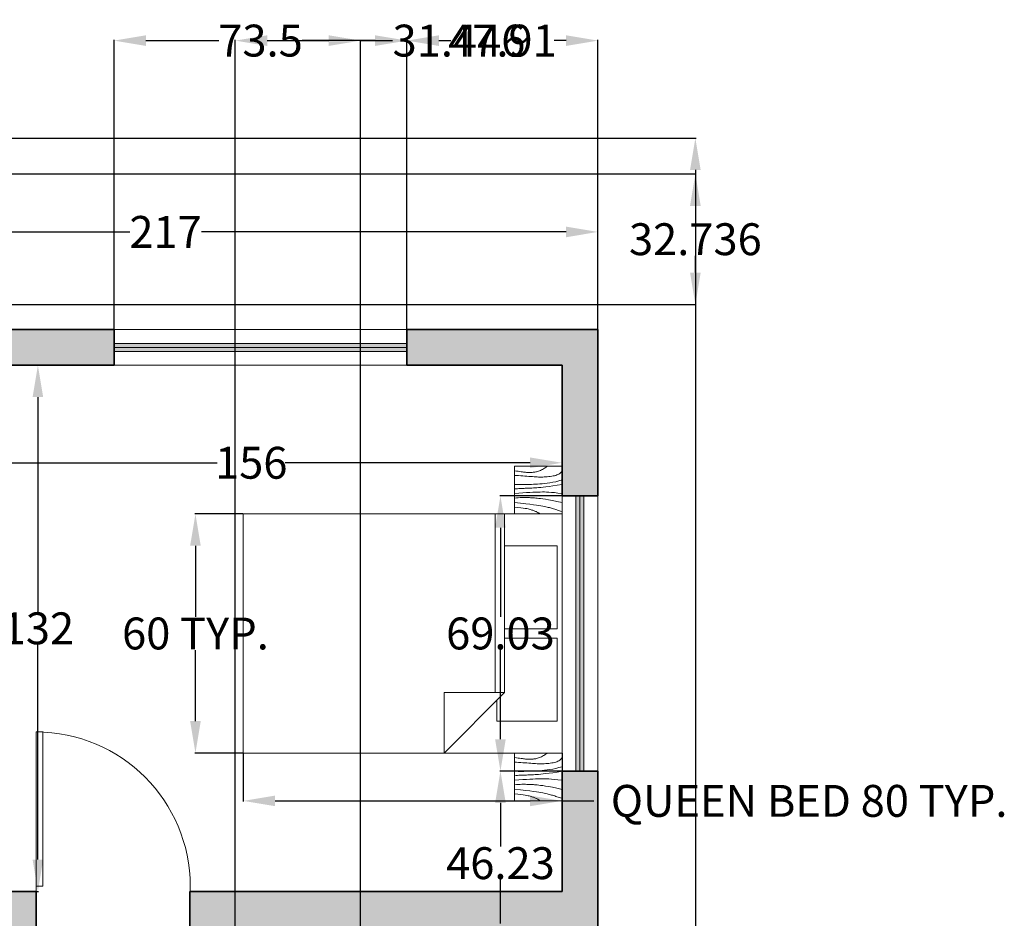
# Model space of a CAD drawing. Units: inches. Extents: x -52 to 678, y 23 to 685.
# Tile 11 of 11: x 431 to 678, y 329 to 555. Entities that reach past the tile are written whole.
import ezdxf

# ---------------------------------------------------------------- set-up
doc = ezdxf.new("R2010")
doc.units = ezdxf.units.IN
doc.header["$MEASUREMENT"] = 0
for name, color, linetype, lineweight in [('A-ANNO-DIMS', 2, 'Continuous', 18), ('A-DOOR', 3, 'Continuous', 18), ('A-FURN', 8, 'Continuous', 18), ('A-GLAZ', 4, 'Continuous', 18), ('A-WALL', 7, 'Continuous', 35)]:
    doc.layers.add(name, color=color, linetype=linetype, lineweight=lineweight)
doc.layers.add('A-GLAZ-PATT', color=18, linetype='Continuous', lineweight=13, true_color=0x000000)
doc.layers.add('A-WALL-PATT', color=18, linetype='Continuous', lineweight=13, true_color=0x000000)
doc.styles.get("Standard").update_dxf_attribs({"font": 'arial.ttf'})
doc.dimstyles.get("Standard").update_dxf_attribs({"dimtxt": 8, "dimasz": 8, "dimexe": 0.18, "dimexo": 0.0625, "dimgap": 0.09, "dimtad": 0, "dimtih": 1, "dimtoh": 1, "dimdec": 0, "dimzin": 0, "dimdsep": 46, "dimlunit": 3, "dimtxsty": 'Standard', "dimcen": 0.09, "dimadec": 0, "dimazin": 0, "dimtfac": 1, "dimtdec": 0, "dimtofl": 0, "dimtmove": 0, "dimatfit": 3, "dimfxl": 1, "dimtolj": 1, "dimtzin": 0, "dimarcsym": 0})

# ---------------------------------------------------------------- blocks, each defined once
blk = doc.blocks.new('Table - Square Woodgrain 42 x 42 in.')
blk.add_line((0, -42), (42, -42))
for points in [[(0, -4), (1.704, -4.2172), (3.2358, -4.4188), (4.615, -4.604), (5.8615, -4.7721), (6.9951, -4.9224), (8.0357, -5.0541), (9.0031, -5.1667), (9.9171, -5.2594), (10.7951, -5.3316), (11.6445, -5.3836), (12.4702, -5.4157), (13.277, -5.4283), (14.0698, -5.4217), (14.8535, -5.3964), (15.6331, -5.3526), (16.4133, -5.2908), (17.1986, -5.2103), (17.9913, -5.1062), (18.793, -4.9727), (19.6056, -4.8038), (20.4307, -4.5937), (21.2701, -4.3365), (22.1256, -4.0262), (22.9989, -3.6571), (23.888, -3.2272), (24.7756, -2.7516), (25.6408, -2.2491), (26.4624, -1.7387), (27.2195, -1.2395), (27.891, -0.7703), (28.456, -0.3501), (28.8934, 0.002)], [(0, -42), (0, 0), (42, 0), (42, -42)], [(0, -8), (1.8203, -8.1001), (3.6741, -8.2149), (5.5411, -8.3408), (7.4011, -8.4741), (9.2339, -8.6112), (11.0193, -8.7484), (12.7371, -8.8821), (14.3671, -9.0086), (15.8954, -9.1246), (17.3337, -9.2278), (18.6997, -9.3159), (20.0116, -9.387), (21.2871, -9.4389), (22.5442, -9.4696), (23.8008, -9.477), (25.0749, -9.459), (26.3791, -9.4137), (27.7049, -9.3403), (29.0383, -9.2382), (30.3655, -9.1068), (31.6728, -8.9455), (32.9461, -8.7535), (34.1717, -8.5304), (35.3358, -8.2756), (36.4268, -7.9863), (37.443, -7.6521), (38.3849, -7.2603), (39.253, -6.7986), (40.048, -6.2542), (40.7705, -5.6147), (41.421, -4.8674), (42, -4)], [(42, -12), (39.1784, -12.8621), (36.4519, -13.5654), (33.8246, -14.1294), (31.3004, -14.5731), (28.8832, -14.9161), (26.577, -15.1775), (24.3858, -15.3768), (22.3136, -15.5332), (20.3622, -15.6632), (18.5254, -15.7718), (16.7947, -15.8612), (15.1618, -15.9338), (13.6183, -15.9916), (12.1558, -16.0369), (10.7659, -16.0718), (9.4403, -16.0987), (8.1703, -16.1191), (6.9461, -16.1325), (5.7577, -16.1377), (4.595, -16.1335), (3.4479, -16.1188), (2.3064, -16.0924), (1.1604, -16.0532), (0, -16)], [(42, -16), (37.6529, -16.7365), (33.8802, -17.329), (30.6179, -17.7961), (27.8015, -18.1561), (25.3668, -18.4275), (23.2497, -18.6288), (21.3859, -18.7785), (19.7111, -18.8949), (18.1693, -18.9939), (16.7375, -19.0795), (15.401, -19.1534), (14.1449, -19.217), (12.9544, -19.2717), (11.8148, -19.3191), (10.7113, -19.3606), (9.6291, -19.3976), (8.5534, -19.4323), (7.47, -19.4689), (6.3643, -19.5122), (5.222, -19.5672), (4.0288, -19.6386), (2.7703, -19.7313), (1.4321, -19.8501), (0, -20)], [(0, -24), (3.9243, -23.6805), (7.4766, -23.4138), (10.6891, -23.1954), (13.5943, -23.0205), (16.2247, -22.8847), (18.6125, -22.7832), (20.7903, -22.7116), (22.7903, -22.6651), (24.6563, -22.642), (26.4764, -22.6507), (28.35, -22.7024), (30.3766, -22.8084), (32.6555, -22.98), (35.2861, -23.2283), (38.3678, -23.5645), (42, -24)], [(42, -32), (37.392, -31.017), (33.4585, -30.2231), (30.1291, -29.5949), (27.3334, -29.109), (25.0009, -28.742), (23.0612, -28.4707), (21.4439, -28.2716), (20.0786, -28.1215), (18.8998, -28.0002), (17.8609, -27.9014), (16.9206, -27.8219), (16.0371, -27.7588), (15.1691, -27.709), (14.2748, -27.6693), (13.3128, -27.6368), (12.2415, -27.6083), (11.0295, -27.5824), (9.6867, -27.5643), (8.233, -27.5608), (6.6884, -27.5787), (5.0728, -27.6248), (3.4062, -27.7058), (1.7086, -27.8286), (0, -28)], [(0, -32), (5.4026, -32.5358), (9.9494, -33.019), (13.7424, -33.4553), (16.8834, -33.8505), (19.4743, -34.2106), (21.6171, -34.5413), (23.4136, -34.8486), (24.9657, -35.1382), (26.3614, -35.4156), (27.6332, -35.6841), (28.7995, -35.9467), (29.8788, -36.2064), (30.8897, -36.4661), (31.8507, -36.7288), (32.7802, -36.9973), (33.6968, -37.2747), (34.6175, -37.5635), (35.5531, -37.8651), (36.5128, -38.1805), (37.506, -38.5108), (38.5421, -38.8568), (39.6302, -39.2197), (40.7797, -39.6004), (42, -40)], [(0, -36), (3.0098, -36.2857), (5.5354, -36.5643), (7.6368, -36.8359), (9.374, -37.1009), (10.807, -37.3597), (11.9957, -37.6126), (13.0002, -37.8599), (13.8804, -38.102), (14.6874, -38.3393), (15.4365, -38.5729), (16.1338, -38.8041), (16.7858, -39.0341), (17.3987, -39.264), (17.9787, -39.4952), (18.5322, -39.7288), (19.0655, -39.9662), (19.5832, -40.2081), (20.0842, -40.4544), (20.5657, -40.7046), (21.0249, -40.9581), (21.459, -41.2144), (21.8653, -41.4731), (22.2409, -41.7335), (22.5831, -41.9951)]]:
    blk.add_lwpolyline(points)
blk = doc.blocks.new('*U14')
for p, q in [((0, 0), (0, -6)), ((40, 0), (40, -6))]:
    blk.add_line(p, q)
blk.add_lwpolyline([(0, 0), (0, 40), (1.75, 40), (1.75, 0)], close=True)
blk.add_arc((0, 0), 40, 0, 90)
blk = doc.blocks.new('Bed - Queen')
for p, q in [((0, -80.00003), (0, 0)), ((0, 0), (59.99999, 0)), ((59.99999, 0), (59.99999, -80.00003)), ((7.99999, -1.2), (28.79998, -1.2)), ((7.99999, -14.4), (7.99999, -1.2)), ((28.79998, -1.2), (28.79998, -14.4)), ((31.19999, -1.2), (51.99999, -1.2)), ((31.19999, -14.4), (31.19999, -1.2)), ((51.99999, -1.2), (51.99999, -16.4)), ((0, -14.4), (44.8, -14.4)), ((59.99999, -29.6), (44.8, -14.4)), ((44.8, -14.4), (44.8, -29.6)), ((44.8, -16.8), (0, -16.8)), ((51.99999, -16.4), (46.79936, -16.4)), ((44.8, -29.6), (59.99999, -29.6)), ((59.99999, -80.00003), (0, -80.00003))]:
    blk.add_line(p, q)
blk = doc.blocks.new('*D19')
at = {"layer": 'A-ANNO-DIMS', "color": 0, "lineweight": -2, "transparency": 16777216}
for p, q in [((486.61, 370.77), (486.61, 358.66)), ((566.61, 370.77), (566.61, 358.66)), ((494.61, 358.84), (558.61, 358.84)), ((566.61, 358.84), (574.61, 358.84))]:
    blk.add_line(p, q, dxfattribs=at)
at = {"layer": 'A-ANNO-DIMS', "color": 0, "transparency": 16777216}
for points in [[(494.61, 360.17), (494.61, 357.5), (486.61, 358.84)], [(558.61, 360.17), (558.61, 357.5), (566.61, 358.84)]]:
    blk.add_solid(points, dxfattribs=at)
at = {"layer": 'Defpoints', "color": 0, "transparency": 16777216}
for p in [(486.61, 370.84), (566.61, 370.84), (566.61, 358.84)]:
    blk.add_point(p, dxfattribs=at)
at = {"layer": 'A-ANNO-DIMS', "color": 0, "transparency": 16777216, "insert": (628.62, 358.84), "char_height": 8, "attachment_point": 5}
blk.add_mtext('\\A1;QUEEN BED 80 TYP.', dxfattribs=at)
blk = doc.blocks.new('*D20')
at = {"layer": 'A-ANNO-DIMS', "color": 0, "lineweight": -2, "transparency": 16777216}
for p, q in [((486.54, 430.84), (474.43, 430.84)), ((474.61, 422.84), (474.61, 405.01)), ((474.61, 378.84), (474.61, 396.66)), ((486.54, 370.84), (474.43, 370.84))]:
    blk.add_line(p, q, dxfattribs=at)
at = {"layer": 'A-ANNO-DIMS', "color": 0, "transparency": 16777216}
for points in [[(473.27, 422.84), (475.94, 422.84), (474.61, 430.84)], [(473.27, 378.84), (475.94, 378.84), (474.61, 370.84)]]:
    blk.add_solid(points, dxfattribs=at)
at = {"layer": 'Defpoints', "color": 0, "transparency": 16777216}
for p in [(486.61, 430.84), (474.61, 370.84), (486.61, 370.84)]:
    blk.add_point(p, dxfattribs=at)
at = {"layer": 'A-ANNO-DIMS', "color": 0, "transparency": 16777216, "insert": (474.61, 400.84), "char_height": 8, "attachment_point": 5}
blk.add_mtext('\\A1;60 TYP.', dxfattribs=at)
blk = doc.blocks.new('*D40')
at = {"layer": 'A-ANNO-DIMS', "color": 0, "lineweight": -2, "transparency": 16777216}
for p, q in [((358.67, 525.13), (600.25, 525.13)), ((600.07, 517.13), (600.07, 293.23)), ((600.07, 61.13), (600.07, 285.02)), ((575.67, 53.13), (600.25, 53.13))]:
    blk.add_line(p, q, dxfattribs=at)
at = {"layer": 'A-ANNO-DIMS', "color": 0, "transparency": 16777216}
for points in [[(598.73, 517.13), (601.4, 517.13), (600.07, 525.13)], [(598.73, 61.13), (601.4, 61.13), (600.07, 53.13)]]:
    blk.add_solid(points, dxfattribs=at)
at = {"layer": 'Defpoints', "color": 0, "transparency": 16777216}
for p in [(358.61, 525.13), (600.07, 525.13), (575.61, 53.13)]:
    blk.add_point(p, dxfattribs=at)
at = {"layer": 'A-ANNO-DIMS', "color": 0, "transparency": 16777216, "insert": (600.07, 289.13), "char_height": 8, "attachment_point": 5}
blk.add_mtext('\\A1;472', dxfattribs=at)
blk = doc.blocks.new('*D43')
at = {"layer": 'A-ANNO-DIMS', "color": 0, "lineweight": -2, "transparency": 16777216}
for p, q in [((358.61, 477.19), (358.61, 501.77)), ((575.61, 477.19), (575.61, 501.77)), ((366.61, 501.59), (458.11, 501.59)), ((567.61, 501.59), (476.1, 501.59))]:
    blk.add_line(p, q, dxfattribs=at)
at = {"layer": 'A-ANNO-DIMS', "color": 0, "transparency": 16777216}
for points in [[(366.61, 502.92), (366.61, 500.25), (358.61, 501.59)], [(567.61, 502.92), (567.61, 500.25), (575.61, 501.59)]]:
    blk.add_solid(points, dxfattribs=at)
at = {"layer": 'Defpoints', "color": 0, "transparency": 16777216}
for p in [(575.61, 501.59), (358.61, 477.13), (575.61, 477.13)]:
    blk.add_point(p, dxfattribs=at)
at = {"layer": 'A-ANNO-DIMS', "color": 0, "transparency": 16777216, "insert": (467.11, 501.59), "char_height": 8, "attachment_point": 5}
blk.add_mtext('\\A1;217', dxfattribs=at)
blk = doc.blocks.new('*D57')
at = {"layer": 'A-ANNO-DIMS', "color": 0, "lineweight": -2, "transparency": 16777216}
for p, q in [((410.61, 468.06), (410.61, 443.49)), ((566.61, 468.06), (566.61, 443.49)), ((418.61, 443.67), (480.06, 443.67)), ((558.61, 443.67), (497.15, 443.67))]:
    blk.add_line(p, q, dxfattribs=at)
at = {"layer": 'A-ANNO-DIMS', "color": 0, "transparency": 16777216}
for points in [[(418.61, 445), (418.61, 442.33), (410.61, 443.67)], [(558.61, 445), (558.61, 442.33), (566.61, 443.67)]]:
    blk.add_solid(points, dxfattribs=at)
at = {"layer": 'Defpoints', "color": 0, "transparency": 16777216}
for p in [(410.61, 468.13), (566.61, 468.13), (410.61, 443.67)]:
    blk.add_point(p, dxfattribs=at)
at = {"layer": 'A-ANNO-DIMS', "color": 0, "transparency": 16777216, "insert": (488.61, 443.67), "char_height": 8, "attachment_point": 5}
blk.add_mtext('\\A1;156', dxfattribs=at)
blk = doc.blocks.new('*D58')
at = {"layer": 'A-ANNO-DIMS', "color": 0, "lineweight": -2, "transparency": 16777216}
for p, q in [((410.67, 468.13), (435.25, 468.13)), ((435.07, 460.13), (435.07, 406.3)), ((435.07, 344.13), (435.07, 397.95)), ((410.67, 336.13), (435.25, 336.13))]:
    blk.add_line(p, q, dxfattribs=at)
at = {"layer": 'A-ANNO-DIMS', "color": 0, "transparency": 16777216}
for points in [[(433.73, 460.13), (436.4, 460.13), (435.07, 468.13)], [(433.73, 344.13), (436.4, 344.13), (435.07, 336.13)]]:
    blk.add_solid(points, dxfattribs=at)
at = {"layer": 'Defpoints', "color": 0, "transparency": 16777216}
for p in [(410.61, 468.13), (410.61, 336.13), (435.07, 336.13)]:
    blk.add_point(p, dxfattribs=at)
at = {"layer": 'A-ANNO-DIMS', "color": 0, "transparency": 16777216, "insert": (435.07, 402.13), "char_height": 8, "attachment_point": 5}
blk.add_mtext('\\A1;132', dxfattribs=at)
blk = doc.blocks.new('*D66')
at = {"layer": 'A-ANNO-DIMS', "color": 0, "lineweight": -2, "transparency": 16777216}
for p, q in [((454.19, 477.19), (454.19, 549.77)), ((462.19, 549.59), (480.47, 549.59)), ((519.69, 549.59), (501.42, 549.59)), ((527.69, 477.19), (527.69, 549.77))]:
    blk.add_line(p, q, dxfattribs=at)
at = {"layer": 'A-ANNO-DIMS', "color": 0, "transparency": 16777216}
for points in [[(462.19, 550.92), (462.19, 548.25), (454.19, 549.59)], [(519.69, 550.92), (519.69, 548.25), (527.69, 549.59)]]:
    blk.add_solid(points, dxfattribs=at)
at = {"layer": 'Defpoints', "color": 0, "transparency": 16777216}
for p in [(527.69, 549.59), (454.19, 477.13), (527.69, 477.13)]:
    blk.add_point(p, dxfattribs=at)
at = {"layer": 'A-ANNO-DIMS', "color": 0, "transparency": 16777216, "insert": (490.94, 549.59), "char_height": 8, "attachment_point": 5}
blk.add_mtext('\\A1;73.5', dxfattribs=at)
blk = doc.blocks.new('*D67')
at = {"layer": 'A-ANNO-DIMS', "color": 0, "lineweight": -2, "transparency": 16777216}
for p, q in [((527.69, 477.19), (527.69, 549.77)), ((535.69, 549.59), (538.67, 549.59)), ((567.61, 549.59), (564.63, 549.59)), ((575.61, 477.19), (575.61, 549.77))]:
    blk.add_line(p, q, dxfattribs=at)
at = {"layer": 'A-ANNO-DIMS', "color": 0, "transparency": 16777216}
for points in [[(535.69, 550.92), (535.69, 548.25), (527.69, 549.59)], [(567.61, 550.92), (567.61, 548.25), (575.61, 549.59)]]:
    blk.add_solid(points, dxfattribs=at)
at = {"layer": 'Defpoints', "color": 0, "transparency": 16777216}
for p in [(575.61, 549.59), (527.69, 477.13), (575.61, 477.13)]:
    blk.add_point(p, dxfattribs=at)
at = {"layer": 'A-ANNO-DIMS', "color": 0, "transparency": 16777216, "insert": (551.65, 549.59), "char_height": 8, "attachment_point": 5}
blk.add_mtext('\\A1;47.91', dxfattribs=at)
blk = doc.blocks.new('*D85')
at = {"layer": 'A-ANNO-DIMS', "color": 0, "lineweight": -2, "transparency": 16777216}
for p, q in [((349.67, 516.13), (600.25, 516.13)), ((600.07, 508.13), (600.07, 503.94)), ((600.07, 491.39), (600.07, 495.58)), ((310.42, 483.39), (600.25, 483.39))]:
    blk.add_line(p, q, dxfattribs=at)
at = {"layer": 'A-ANNO-DIMS', "color": 0, "transparency": 16777216}
for points in [[(598.73, 508.13), (601.4, 508.13), (600.07, 516.13)], [(598.73, 491.39), (601.4, 491.39), (600.07, 483.39)]]:
    blk.add_solid(points, dxfattribs=at)
at = {"layer": 'Defpoints', "color": 0, "transparency": 16777216}
for p in [(349.61, 516.13), (600.07, 516.13), (310.36, 483.39)]:
    blk.add_point(p, dxfattribs=at)
at = {"layer": 'A-ANNO-DIMS', "color": 0, "transparency": 16777216, "insert": (600.07, 499.76), "char_height": 8, "attachment_point": 5}
blk.add_mtext('\\A1;32.736', dxfattribs=at)
blk = doc.blocks.new('*D94')
at = {"layer": 'A-ANNO-DIMS', "color": 0, "lineweight": -2, "transparency": 16777216}
for p, q in [((575.54, 366.32), (550.97, 366.32)), ((551.15, 358.32), (551.15, 347.38)), ((551.15, 328.09), (551.15, 339.03)), ((575.54, 320.09), (550.97, 320.09))]:
    blk.add_line(p, q, dxfattribs=at)
at = {"layer": 'A-ANNO-DIMS', "color": 0, "transparency": 16777216}
for points in [[(549.81, 358.32), (552.48, 358.32), (551.15, 366.32)], [(549.81, 328.09), (552.48, 328.09), (551.15, 320.09)]]:
    blk.add_solid(points, dxfattribs=at)
at = {"layer": 'Defpoints', "color": 0, "transparency": 16777216}
for p in [(551.15, 366.32), (575.61, 366.32), (575.61, 320.09)]:
    blk.add_point(p, dxfattribs=at)
at = {"layer": 'A-ANNO-DIMS', "color": 0, "transparency": 16777216, "insert": (551.15, 343.21), "char_height": 8, "attachment_point": 5}
blk.add_mtext('\\A1;46.23', dxfattribs=at)
blk = doc.blocks.new('*D95')
at = {"layer": 'A-ANNO-DIMS', "color": 0, "lineweight": -2, "transparency": 16777216}
for p, q in [((575.54, 435.35), (550.97, 435.35)), ((551.15, 427.35), (551.15, 405.01)), ((551.15, 374.32), (551.15, 396.66)), ((575.54, 366.32), (550.97, 366.32))]:
    blk.add_line(p, q, dxfattribs=at)
at = {"layer": 'A-ANNO-DIMS', "color": 0, "transparency": 16777216}
for points in [[(549.81, 427.35), (552.48, 427.35), (551.15, 435.35)], [(549.81, 374.32), (552.48, 374.32), (551.15, 366.32)]]:
    blk.add_solid(points, dxfattribs=at)
at = {"layer": 'Defpoints', "color": 0, "transparency": 16777216}
for p in [(551.15, 435.35), (575.61, 435.35), (575.61, 366.32)]:
    blk.add_point(p, dxfattribs=at)
at = {"layer": 'A-ANNO-DIMS', "color": 0, "transparency": 16777216, "insert": (551.15, 400.84), "char_height": 8, "attachment_point": 5}
blk.add_mtext('\\A1;69.03', dxfattribs=at)
blk = doc.blocks.new('*D99')
at = {"layer": 'A-ANNO-DIMS', "color": 0, "lineweight": -2, "transparency": 16777216}
for p, q in [((484.61, 275.19), (484.61, 549.77)), ((492.61, 549.59), (508.05, 549.59)), ((516.05, 279.19), (516.05, 549.77)), ((516.05, 549.59), (524.05, 549.59))]:
    blk.add_line(p, q, dxfattribs=at)
at = {"layer": 'A-ANNO-DIMS', "color": 0, "transparency": 16777216}
for points in [[(492.61, 550.92), (492.61, 548.25), (484.61, 549.59)], [(508.05, 550.92), (508.05, 548.25), (516.05, 549.59)]]:
    blk.add_solid(points, dxfattribs=at)
at = {"layer": 'Defpoints', "color": 0, "transparency": 16777216}
for p in [(516.05, 549.59), (516.05, 279.13), (484.61, 275.13)]:
    blk.add_point(p, dxfattribs=at)
at = {"layer": 'A-ANNO-DIMS', "color": 0, "transparency": 16777216, "insert": (540.74, 549.59), "char_height": 8, "attachment_point": 5}
blk.add_mtext('\\A1;31.446', dxfattribs=at)

msp = doc.modelspace()

# ---------------------------------------------------------------- hatches: boundary and pattern name
at = {"layer": 'A-GLAZ-PATT'}
h = msp.add_hatch(color=256, dxfattribs=at)
h.dxf.hatch_style = 1
h.paths.add_polyline_path([(454.1942, 473.6267), (454.1942, 472.6267), (527.6932, 472.6267), (527.6932, 473.6267)])
h = msp.add_hatch(color=256, dxfattribs=at)
h.dxf.hatch_style = 1
h.paths.add_polyline_path([(454.1942, 472.6267), (454.1942, 471.6267), (527.6932, 471.6267), (527.6932, 472.6267)])
h = msp.add_hatch(color=256, dxfattribs=at)
h.dxf.hatch_style = 1
h.paths.add_polyline_path([(570.1053, 366.3195), (571.1053, 366.3195), (571.1053, 435.3512), (570.1053, 435.3512)])
h = msp.add_hatch(color=256, dxfattribs=at)
h.dxf.hatch_style = 1
h.paths.add_polyline_path([(572.1053, 435.3512), (571.1053, 435.3512), (571.1053, 366.3195), (572.1053, 366.3195)])
at = {"layer": 'A-WALL-PATT'}
h = msp.add_hatch(color=256, dxfattribs=at)
h.dxf.hatch_style = 1
h.paths.add_polyline_path([(349.6053, 340.107), (349.6053, 327.1267), (410.6053, 327.1267), (434.6053, 327.1267), (434.6053, 336.1267), (410.6053, 336.1267), (410.6053, 340.107), (410.6053, 363.4905), (406.6053, 363.4905), (406.6053, 340.107), (406.6053, 336.1267), (358.6053, 336.1267), (358.6053, 340.107), (358.6053, 392.1267), (382.6053, 392.1267), (382.6053, 396.1267), (358.6053, 396.1267), (358.6053, 468.1267), (372.5751, 468.1267), (372.5751, 477.1267), (358.6053, 477.1267), (358.6053, 525.1267), (341.0247, 525.1267), (341.0247, 516.1267), (349.6053, 516.1267)])
h = msp.add_hatch(color=256, dxfattribs=at)
h.dxf.hatch_style = 1
h.paths.add_polyline_path([(410.6053, 477.1267), (406.6053, 477.1267), (406.6053, 392.1267), (410.6053, 392.1267), (410.6053, 468.1267), (454.1942, 468.1267), (454.1942, 477.1267)])
h = msp.add_hatch(color=256, dxfattribs=at)
h.dxf.hatch_style = 1
h.paths.add_polyline_path([(527.6932, 477.1267), (527.6932, 468.1267), (566.6053, 468.1267), (566.6053, 435.3512), (575.6053, 435.3512), (575.6053, 477.1267)])
h = msp.add_hatch(color=256, dxfattribs=at)
h.dxf.hatch_style = 1
h.paths.add_polyline_path([(575.6053, 366.3195), (566.6053, 366.3195), (566.6053, 336.1267), (473.2028, 336.1267), (473.2028, 327.1267), (480.6053, 327.1267), (480.6053, 275.1267), (484.6053, 275.1267), (484.6053, 327.1267), (566.6053, 327.1267), (566.6053, 320.0909), (575.6053, 320.0909)])

# ---------------------------------------------------------------- linework, layer by layer
at = {"layer": 'A-GLAZ'}
for p, q in [((454.1942, 477.1267), (527.6932, 477.1267)), ((454.1942, 473.6267), (527.6932, 473.6267)), ((454.1942, 472.6267), (527.6932, 472.6267)), ((454.1942, 471.6267), (527.6932, 471.6267)), ((454.1942, 468.1267), (527.6932, 468.1267)), ((566.6053, 435.3512), (566.6053, 366.3195)), ((570.1053, 435.3512), (570.1053, 366.3195)), ((571.1053, 435.3512), (571.1053, 366.3195)), ((572.1053, 435.3512), (572.1053, 366.3195)), ((575.6053, 435.3512), (575.6053, 366.3195))]:
    msp.add_line(p, q, dxfattribs=at)
at = {"layer": 'A-WALL'}
for p, q in [((410.6053, 477.1267), (454.1942, 477.1267)), ((454.1942, 477.1267), (454.1942, 468.1267)), ((527.6932, 468.1267), (527.6932, 477.1267)), ((527.6932, 477.1267), (575.6053, 477.1267)), ((575.6053, 435.3512), (575.6053, 477.1267)), ((410.6053, 468.1267), (454.1942, 468.1267)), ((527.6932, 468.1267), (566.6053, 468.1267)), ((566.6053, 435.3512), (566.6053, 468.1267)), ((575.6053, 435.3512), (566.6053, 435.3512)), ((566.6053, 336.1267), (566.6053, 366.3195)), ((566.6053, 366.3195), (575.6053, 366.3195)), ((575.6053, 320.0909), (575.6053, 366.3195)), ((410.6053, 336.1267), (434.6053, 336.1267)), ((434.6053, 327.1267), (434.6053, 336.1267)), ((473.2028, 327.1267), (473.2028, 336.1267)), ((473.2028, 336.1267), (566.6053, 336.1267))]:
    msp.add_line(p, q, dxfattribs=at)

# ---------------------------------------------------------------- block references
at = {"layer": 'A-DOOR', "xscale": 0.9672617031714532, "yscale": 0.9672617031714532, "zscale": 0.9672617031714532}
msp.add_blockref('*U14', (434.6053, 337.4303), dxfattribs=at)
at = {"layer": 'A-FURN', "xscale": 0.2844588312427021, "yscale": 0.2844588312427021, "zscale": 0.2844588312427021}
for p in [(554.658, 442.7826), (554.658, 370.8353)]:
    msp.add_blockref('Table - Square Woodgrain 42 x 42 in.', p, dxfattribs=at)
at = {"layer": 'A-FURN', "rotation": 270}
msp.add_blockref('Bed - Queen', (566.6053, 430.8353), dxfattribs=at)

# ---------------------------------------------------------------- dimensions: what is measured, and where the dimension line sits
at = {"layer": 'A-ANNO-DIMS'}
for base, p1, p2, override, picture, middle in [((527.6932, 549.5867), (454.1942, 477.1267), (527.6932, 477.1267), {"dimdec": 1, "dimlfac": 1, "dimrnd": 0, "dimzin": 0, "dimdsep": 46, "dimlunit": 2}, '*D66', (490.9437, 549.5867)), ((516.0511, 549.5867), (484.6053, 275.1267), (516.0511, 279.1267), {"dimdec": 3, "dimlfac": 1, "dimrnd": 0, "dimzin": 0, "dimdsep": 46, "dimlunit": 2}, '*D99', (540.7414, 549.5867)), ((575.6053, 549.5867), (527.6932, 477.1267), (575.6053, 477.1267), {"dimdec": 2, "dimlfac": 1, "dimrnd": 0, "dimzin": 0, "dimdsep": 46, "dimlunit": 2}, '*D67', (551.6492, 549.5867)), ((575.6053, 501.5867), (358.6053, 477.1267), (575.6053, 477.1267), {"dimdec": 0, "dimlfac": 1, "dimrnd": 0, "dimzin": 0, "dimdsep": 46, "dimlunit": 2}, '*D43', (467.1053, 501.5867))]:
    dim = msp.add_linear_dim(base=base, p1=p1, p2=p2, dimstyle='Standard', override=override, dxfattribs=at)
    dim.commit()
    dim.dimension.update_dxf_attribs({"geometry": picture, "text_midpoint": middle})
for base, p1, p2, angle, override, picture, middle in [((600.0653, 525.1267), (575.6053, 53.1267), (358.6053, 525.1267), 90, {"dimdec": 0, "dimlfac": 1, "dimrnd": 0, "dimzin": 0, "dimdsep": 46, "dimlunit": 2}, '*D40', (600.0653, 289.1267)), ((600.0653, 516.1267), (310.3563, 483.3905), (349.6053, 516.1267), 90, {"dimdec": 3, "dimlfac": 1, "dimrnd": 0, "dimzin": 0, "dimdsep": 46, "dimlunit": 2}, '*D85', (600.0653, 499.7586)), ((410.6053, 443.6667), (566.6053, 468.1267), (410.6053, 468.1267), 180, {"dimdec": 0, "dimlfac": 1, "dimrnd": 0, "dimzin": 0, "dimdsep": 46, "dimlunit": 2}, '*D57', (488.6053, 443.6667)), ((435.0653, 336.1267), (410.6053, 468.1267), (410.6053, 336.1267), 270, {"dimdec": 0, "dimlfac": 1, "dimrnd": 0, "dimzin": 0, "dimdsep": 46, "dimlunit": 2}, '*D58', (435.0653, 402.1267)), ((551.1453, 435.3512), (575.6053, 366.3195), (575.6053, 435.3512), 90, {"dimdec": 2, "dimlfac": 1, "dimrnd": 0, "dimzin": 0, "dimdsep": 46, "dimlunit": 2}, '*D95', (551.1453, 400.8353)), ((551.1453, 366.3195), (575.6053, 320.0909), (575.6053, 366.3195), 90, {"dimdec": 2, "dimlfac": 1, "dimrnd": 0, "dimzin": 0, "dimdsep": 46, "dimlunit": 2}, '*D94', (551.1453, 343.2052))]:
    dim = msp.add_linear_dim(base=base, p1=p1, p2=p2, angle=angle, dimstyle='Standard', override=override, dxfattribs=at)
    dim.commit()
    dim.dimension.update_dxf_attribs({"geometry": picture, "text_midpoint": middle})
dim = msp.add_linear_dim(base=(474.6052, 370.8353), p1=(486.6052, 430.8353), p2=(486.6052, 370.8353), angle=270, text='<> TYP.', dimstyle='Standard', override={"dimdec": 0, "dimlfac": 1, "dimrnd": 0, "dimzin": 0, "dimdsep": 46, "dimlunit": 2}, dxfattribs=at)
dim.commit()
dim.dimension.update_dxf_attribs({"geometry": '*D20', "text_midpoint": (474.6052, 400.8353)})
dim = msp.add_linear_dim(base=(566.6053, 358.8353), p1=(486.6052, 370.8353), p2=(566.6053, 370.8353), text='QUEEN BED <> TYP.', dimstyle='Standard', override={"dimdec": 0, "dimlfac": 1, "dimrnd": 0, "dimzin": 0, "dimdsep": 46, "dimlunit": 2}, dxfattribs=at)
dim.commit()
dim.dimension.update_dxf_attribs({"geometry": '*D19', "text_midpoint": (628.6243, 358.8353)})

doc.saveas('drawing.dxf')
